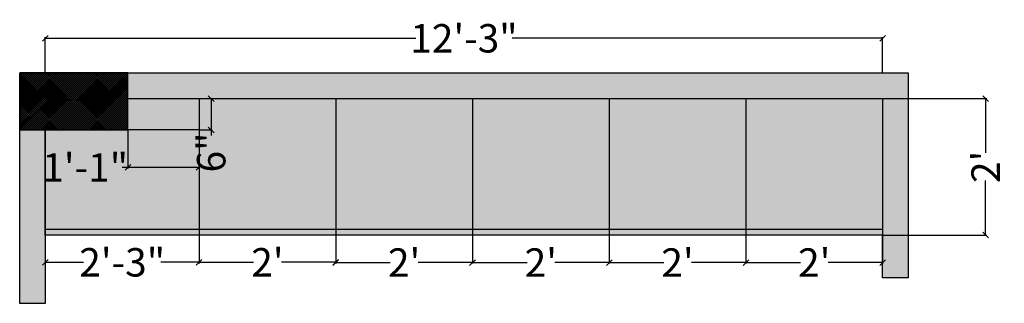
# Model space of a CAD drawing. Units: inches. Extents: x 1441 to 1633, y 516 to 722.
# Tile 2 of 2: x 1460 to 1633, y 673 to 722. Entities that reach past the tile are written whole.
import ezdxf

# ---------------------------------------------------------------- set-up
doc = ezdxf.new("R2010")
doc.units = ezdxf.units.IN
doc.header["$LTSCALE"] = 2
doc.header["$MEASUREMENT"] = 0
for name, color, linetype, lineweight in [('A-ANNO-DIMS', 2, 'Continuous', 18), ('A-FURN', 7, 'Continuous', 25), ('A-FURN-PATT', 252, 'Continuous', 13)]:
    doc.layers.add(name, color=color, linetype=linetype, lineweight=lineweight)
doc.styles.get("Standard").update_dxf_attribs({"font": 'arial.ttf'})
doc.dimstyles.get("Standard").update_dxf_attribs({"dimtxt": 5, "dimasz": 1, "dimexe": 0.18, "dimexo": 0.0625, "dimgap": 0.09, "dimtad": 0, "dimdec": 0, "dimzin": 0, "dimdsep": 46, "dimlunit": 4, "dimtxsty": 'Standard', "dimblk": 'OBLIQUE', "dimcen": 0.09, "dimadec": 0, "dimazin": 0, "dimtfac": 1, "dimtdec": 0, "dimtofl": 0, "dimtmove": 0, "dimatfit": 3, "dimldrblk": 'OBLIQUE', "dimfxl": 1, "dimtolj": 1, "dimtzin": 0, "dimarcsym": 1})

# ---------------------------------------------------------------- blocks, each defined once
blk = doc.blocks.new('_Oblique')
at = {"color": 0, "linetype": 'ByBlock', "lineweight": -2}
blk.add_line((-0.5, -0.5), (0.5, 0.5), dxfattribs=at)
blk = doc.blocks.new('*D2')
at = {"layer": 'A-ANNO-DIMS', "color": 0, "lineweight": -2, "transparency": 16777216}
for p, q in [((1464.16, 713.06), (1464.16, 719.27)), ((1611.16, 713.06), (1611.16, 719.27)), ((1464.16, 719.09), (1529.22, 719.09)), ((1611.16, 719.09), (1546.11, 719.09))]:
    blk.add_line(p, q, dxfattribs=at)
at = {"layer": 'Defpoints', "color": 0, "transparency": 16777216}
for p in [(1611.16, 719.09), (1464.16, 713), (1611.16, 713)]:
    blk.add_point(p, dxfattribs=at)
at = {"layer": 'A-ANNO-DIMS', "color": 0, "lineweight": -2, "transparency": 16777216, "rotation": 180}
blk.add_blockref('_Oblique', (1464.16, 719.09), dxfattribs=at)
at = {"layer": 'A-ANNO-DIMS', "color": 0, "lineweight": -2, "transparency": 16777216}
blk.add_blockref('_Oblique', (1611.16, 719.09), dxfattribs=at)
at = {"layer": 'A-ANNO-DIMS', "color": 0, "transparency": 16777216, "insert": (1537.66, 719.09), "char_height": 5, "attachment_point": 5}
blk.add_mtext('\\A1;12\'-3"', dxfattribs=at)
blk = doc.blocks.new('*D25')
at = {"layer": 'A-ANNO-DIMS', "color": 0, "lineweight": -2, "transparency": 16777216}
for p, q in [((1464.16, 685.44), (1464.16, 679.53)), ((1491.16, 685.44), (1491.16, 679.53)), ((1464.16, 679.71), (1470.88, 679.71)), ((1491.16, 679.71), (1484.44, 679.71))]:
    blk.add_line(p, q, dxfattribs=at)
at = {"layer": 'Defpoints', "color": 0, "transparency": 16777216}
for p in [(1464.16, 685.5), (1491.16, 685.5), (1491.16, 679.71)]:
    blk.add_point(p, dxfattribs=at)
at = {"layer": 'A-ANNO-DIMS', "color": 0, "lineweight": -2, "transparency": 16777216, "rotation": 180}
blk.add_blockref('_Oblique', (1464.16, 679.71), dxfattribs=at)
at = {"layer": 'A-ANNO-DIMS', "color": 0, "lineweight": -2, "transparency": 16777216}
blk.add_blockref('_Oblique', (1491.16, 679.71), dxfattribs=at)
at = {"layer": 'A-ANNO-DIMS', "color": 0, "transparency": 16777216, "insert": (1477.66, 679.71), "char_height": 5, "attachment_point": 5}
blk.add_mtext('\\A1;2\'-3"', dxfattribs=at)
blk = doc.blocks.new('*D26')
at = {"layer": 'A-ANNO-DIMS', "color": 0, "lineweight": -2, "transparency": 16777216}
for p, q in [((1515.16, 685.44), (1515.16, 679.53)), ((1491.16, 679.78), (1491.16, 679.89)), ((1491.16, 679.71), (1500.73, 679.71)), ((1515.16, 679.71), (1505.6, 679.71))]:
    blk.add_line(p, q, dxfattribs=at)
at = {"layer": 'Defpoints', "color": 0, "transparency": 16777216}
for p in [(1515.16, 685.5), (1491.16, 679.71), (1515.16, 679.71)]:
    blk.add_point(p, dxfattribs=at)
at = {"layer": 'A-ANNO-DIMS', "color": 0, "lineweight": -2, "transparency": 16777216, "rotation": 180}
blk.add_blockref('_Oblique', (1491.16, 679.71), dxfattribs=at)
at = {"layer": 'A-ANNO-DIMS', "color": 0, "lineweight": -2, "transparency": 16777216}
blk.add_blockref('_Oblique', (1515.16, 679.71), dxfattribs=at)
at = {"layer": 'A-ANNO-DIMS', "color": 0, "transparency": 16777216, "insert": (1503.16, 679.71), "char_height": 5, "attachment_point": 5}
blk.add_mtext("\\A1;2'", dxfattribs=at)
blk = doc.blocks.new('*D27')
at = {"layer": 'A-ANNO-DIMS', "color": 0, "lineweight": -2, "transparency": 16777216}
for p, q in [((1539.16, 685.44), (1539.16, 679.49)), ((1515.16, 679.67), (1524.73, 679.67)), ((1515.16, 679.65), (1515.16, 679.49)), ((1539.16, 679.67), (1529.6, 679.67))]:
    blk.add_line(p, q, dxfattribs=at)
at = {"layer": 'Defpoints', "color": 0, "transparency": 16777216}
for p in [(1539.16, 685.5), (1515.16, 679.71), (1515.16, 679.67)]:
    blk.add_point(p, dxfattribs=at)
at = {"layer": 'A-ANNO-DIMS', "color": 0, "lineweight": -2, "transparency": 16777216, "rotation": 180}
blk.add_blockref('_Oblique', (1515.16, 679.67), dxfattribs=at)
at = {"layer": 'A-ANNO-DIMS', "color": 0, "lineweight": -2, "transparency": 16777216}
blk.add_blockref('_Oblique', (1539.16, 679.67), dxfattribs=at)
at = {"layer": 'A-ANNO-DIMS', "color": 0, "transparency": 16777216, "insert": (1527.16, 679.67), "char_height": 5, "attachment_point": 5}
blk.add_mtext("\\A1;2'", dxfattribs=at)
blk = doc.blocks.new('*D28')
at = {"layer": 'A-ANNO-DIMS', "color": 0, "lineweight": -2, "transparency": 16777216}
for p, q in [((1539.16, 685.44), (1539.16, 679.49)), ((1563.16, 685.44), (1563.16, 679.49)), ((1539.16, 679.67), (1548.73, 679.67)), ((1563.16, 679.67), (1553.6, 679.67))]:
    blk.add_line(p, q, dxfattribs=at)
at = {"layer": 'Defpoints', "color": 0, "transparency": 16777216}
for p in [(1539.16, 685.5), (1563.16, 685.5), (1563.16, 679.67)]:
    blk.add_point(p, dxfattribs=at)
at = {"layer": 'A-ANNO-DIMS', "color": 0, "lineweight": -2, "transparency": 16777216, "rotation": 180}
blk.add_blockref('_Oblique', (1539.16, 679.67), dxfattribs=at)
at = {"layer": 'A-ANNO-DIMS', "color": 0, "lineweight": -2, "transparency": 16777216}
blk.add_blockref('_Oblique', (1563.16, 679.67), dxfattribs=at)
at = {"layer": 'A-ANNO-DIMS', "color": 0, "transparency": 16777216, "insert": (1551.16, 679.67), "char_height": 5, "attachment_point": 5}
blk.add_mtext("\\A1;2'", dxfattribs=at)
blk = doc.blocks.new('*D29')
at = {"layer": 'A-ANNO-DIMS', "color": 0, "lineweight": -2, "transparency": 16777216}
for p, q in [((1563.16, 685.44), (1563.16, 679.49)), ((1587.16, 685.44), (1587.16, 679.49)), ((1563.16, 679.67), (1572.73, 679.67)), ((1587.16, 679.67), (1577.6, 679.67))]:
    blk.add_line(p, q, dxfattribs=at)
at = {"layer": 'Defpoints', "color": 0, "transparency": 16777216}
for p in [(1563.16, 685.5), (1587.16, 685.5), (1587.16, 679.67)]:
    blk.add_point(p, dxfattribs=at)
at = {"layer": 'A-ANNO-DIMS', "color": 0, "lineweight": -2, "transparency": 16777216, "rotation": 180}
blk.add_blockref('_Oblique', (1563.16, 679.67), dxfattribs=at)
at = {"layer": 'A-ANNO-DIMS', "color": 0, "lineweight": -2, "transparency": 16777216}
blk.add_blockref('_Oblique', (1587.16, 679.67), dxfattribs=at)
at = {"layer": 'A-ANNO-DIMS', "color": 0, "transparency": 16777216, "insert": (1575.16, 679.67), "char_height": 5, "attachment_point": 5}
blk.add_mtext("\\A1;2'", dxfattribs=at)
blk = doc.blocks.new('*D30')
at = {"layer": 'A-ANNO-DIMS', "color": 0, "lineweight": -2, "transparency": 16777216}
for p, q in [((1587.16, 685.44), (1587.16, 679.49)), ((1611.16, 685.44), (1611.16, 679.49)), ((1587.16, 679.67), (1596.73, 679.67)), ((1611.16, 679.67), (1601.6, 679.67))]:
    blk.add_line(p, q, dxfattribs=at)
at = {"layer": 'Defpoints', "color": 0, "transparency": 16777216}
for p in [(1587.16, 685.5), (1611.16, 685.5), (1611.16, 679.67)]:
    blk.add_point(p, dxfattribs=at)
at = {"layer": 'A-ANNO-DIMS', "color": 0, "lineweight": -2, "transparency": 16777216, "rotation": 180}
blk.add_blockref('_Oblique', (1587.16, 679.67), dxfattribs=at)
at = {"layer": 'A-ANNO-DIMS', "color": 0, "lineweight": -2, "transparency": 16777216}
blk.add_blockref('_Oblique', (1611.16, 679.67), dxfattribs=at)
at = {"layer": 'A-ANNO-DIMS', "color": 0, "transparency": 16777216, "insert": (1599.16, 679.67), "char_height": 5, "attachment_point": 5}
blk.add_mtext("\\A1;2'", dxfattribs=at)
blk = doc.blocks.new('*D31')
at = {"layer": 'A-ANNO-DIMS', "color": 0, "lineweight": -2, "transparency": 16777216}
for p, q in [((1611.23, 708.5), (1629.43, 708.5)), ((1629.25, 708.5), (1629.25, 698.93)), ((1629.25, 684.5), (1629.25, 694.07)), ((1611.23, 684.5), (1629.43, 684.5))]:
    blk.add_line(p, q, dxfattribs=at)
at = {"layer": 'Defpoints', "color": 0, "transparency": 16777216}
for p in [(1611.16, 708.5), (1611.16, 684.5), (1629.25, 684.5)]:
    blk.add_point(p, dxfattribs=at)
at = {"layer": 'A-ANNO-DIMS', "color": 0, "lineweight": -2, "transparency": 16777216}
for p, rotation in [((1629.25, 708.5), 90), ((1629.25, 684.5), 270)]:
    blk.add_blockref('_Oblique', p, dxfattribs=dict(at, rotation=rotation))
at = {"layer": 'A-ANNO-DIMS', "color": 0, "transparency": 16777216, "insert": (1629.25, 696.5), "char_height": 5, "attachment_point": 5, "rotation": 90}
blk.add_mtext("\\A1;2'", dxfattribs=at)
blk = doc.blocks.new('*D32')
at = {"layer": 'A-ANNO-DIMS', "color": 0, "lineweight": -2, "transparency": 16777216}
for p, q in [((1478.66, 702.94), (1478.66, 696.21)), ((1491.16, 702.94), (1491.16, 696.21)), ((1478.66, 696.39), (1477.66, 696.39)), ((1491.16, 696.39), (1478.66, 696.39))]:
    blk.add_line(p, q, dxfattribs=at)
at = {"layer": 'Defpoints', "color": 0, "transparency": 16777216}
for p in [(1478.66, 703), (1491.16, 703), (1478.66, 696.39)]:
    blk.add_point(p, dxfattribs=at)
at = {"layer": 'A-ANNO-DIMS', "color": 0, "lineweight": -2, "transparency": 16777216, "rotation": 180}
blk.add_blockref('_Oblique', (1478.66, 696.39), dxfattribs=at)
at = {"layer": 'A-ANNO-DIMS', "color": 0, "lineweight": -2, "transparency": 16777216}
blk.add_blockref('_Oblique', (1491.16, 696.39), dxfattribs=at)
at = {"layer": 'A-ANNO-DIMS', "color": 0, "transparency": 16777216, "insert": (1471.16, 696.39), "char_height": 5, "attachment_point": 5}
blk.add_mtext('\\A1;1\'-1"', dxfattribs=at)
blk = doc.blocks.new('*D33')
at = {"layer": 'A-ANNO-DIMS', "color": 0, "lineweight": -2, "transparency": 16777216}
for p, q in [((1491.23, 708.5), (1493.46, 708.5)), ((1493.28, 708.5), (1493.28, 703)), ((1491.23, 703), (1493.46, 703)), ((1493.28, 703), (1493.28, 702))]:
    blk.add_line(p, q, dxfattribs=at)
at = {"layer": 'Defpoints', "color": 0, "transparency": 16777216}
for p in [(1491.16, 708.5), (1491.16, 703), (1493.28, 703)]:
    blk.add_point(p, dxfattribs=at)
at = {"layer": 'A-ANNO-DIMS', "color": 0, "lineweight": -2, "transparency": 16777216}
for p, rotation in [((1493.28, 708.5), 90), ((1493.28, 703), 270)]:
    blk.add_blockref('_Oblique', p, dxfattribs=dict(at, rotation=rotation))
at = {"layer": 'A-ANNO-DIMS', "color": 0, "transparency": 16777216, "insert": (1493.28, 699.02), "char_height": 5, "attachment_point": 5, "rotation": 90}
blk.add_mtext('\\A1;6"', dxfattribs=at)

msp = doc.modelspace()

# ---------------------------------------------------------------- hatches: boundary and pattern name
at = {"layer": 'A-FURN-PATT'}
h = msp.add_hatch(dxfattribs=at)
h.set_pattern_fill('ANSI37', color=256, scale=2)
h.set_pattern_definition([(45, (43.05178, -183.31212), (-0.176776695, 0.176776695), []), (135, (43.05178, -183.31212), (-0.176776695, -0.176776695), [])])
h.paths.add_polyline_path([(1478.66, 703), (1478.66, 713), (1459.66, 713), (1459.66, 703)])
h = msp.add_hatch(color=256, dxfattribs=at)
h.dxf.hatch_style = 1
h.paths.add_polyline_path([(1611.16, 708.5), (1611.16, 684.5), (1611.16, 677), (1615.66, 677), (1615.66, 713), (1611.16, 713), (1478.66, 713), (1478.66, 708.5)])
h.paths.add_polyline_path([(1464.16, 703), (1459.66, 703), (1459.66, 672.5), (1464.16, 672.5), (1464.16, 684.5)])
h = msp.add_hatch(color=256, dxfattribs=at)
h.dxf.hatch_style = 1
h.paths.add_polyline_path([(1491.16, 703), (1478.66, 703), (1464.16, 703), (1464.16, 685.5), (1491.16, 685.5)])
h.paths.add_polyline_path([(1491.16, 708.5), (1478.66, 708.5), (1478.66, 703), (1491.16, 703)])
h.paths.add_polyline_path([(1462.74, 695.19), (1479.15, 695.19), (1479.15, 705.49), (1462.74, 705.49)], flags=9)
h = msp.add_hatch(color=256, dxfattribs=at)
h.dxf.hatch_style = 1
h.paths.add_polyline_path([(1491.16, 708.5), (1478.66, 708.5), (1478.66, 703), (1491.16, 703)])
h.paths.add_polyline_path([(1491.16, 703), (1478.66, 703), (1464.16, 703), (1464.16, 685.5), (1491.16, 685.5)])
h.paths.add_polyline_path([(1515.16, 708.5), (1491.16, 708.5), (1491.16, 703), (1491.16, 685.5), (1515.16, 685.5)])
h.paths.add_polyline_path([(1539.16, 708.5), (1515.16, 708.5), (1515.16, 685.5), (1539.16, 685.5)])
h.paths.add_polyline_path([(1563.16, 708.5), (1539.16, 708.5), (1539.16, 685.5), (1563.16, 685.5)])
h.paths.add_polyline_path([(1587.16, 708.5), (1563.16, 708.5), (1563.16, 685.5), (1587.16, 685.5)])
h.paths.add_polyline_path([(1611.16, 708.5), (1587.16, 708.5), (1587.16, 685.5), (1611.16, 685.5)])
h.paths.add_polyline_path([(1611.16, 685.5), (1587.16, 685.5), (1587.16, 684.5), (1611.16, 684.5)])
h.paths.add_polyline_path([(1587.16, 685.5), (1563.16, 685.5), (1563.16, 684.5), (1587.16, 684.5)])
h.paths.add_polyline_path([(1563.16, 685.5), (1539.16, 685.5), (1539.16, 684.5), (1563.16, 684.5)])
h.paths.add_polyline_path([(1539.16, 685.5), (1515.16, 685.5), (1515.16, 684.5), (1539.16, 684.5)])
h.paths.add_polyline_path([(1515.16, 685.5), (1491.16, 685.5), (1491.16, 684.5), (1515.16, 684.5)])
h.paths.add_polyline_path([(1491.16, 685.5), (1464.16, 685.5), (1464.16, 684.5), (1491.16, 684.5)])

# ---------------------------------------------------------------- linework, layer by layer
at = {"layer": 'A-FURN'}
for p, q in [((1459.66, 708.5), (1459.66, 713)), ((1459.66, 713), (1464.16, 713)), ((1464.16, 713), (1611.16, 713)), ((1611.16, 713), (1615.66, 713)), ((1615.66, 713), (1615.66, 677)), ((1459.66, 672.5), (1459.66, 708.5)), ((1478.66, 708.5), (1611.16, 708.5)), ((1491.16, 708.5), (1491.16, 684.5)), ((1515.16, 708.5), (1515.16, 684.5)), ((1539.16, 708.5), (1539.16, 684.5)), ((1563.16, 708.5), (1563.16, 684.5)), ((1587.16, 708.5), (1587.16, 684.5)), ((1611.16, 708.5), (1611.16, 684.5)), ((1464.16, 684.5), (1464.16, 703)), ((1464.16, 703), (1464.16, 684.5)), ((1611.16, 685.5), (1464.16, 685.5)), ((1611.16, 684.5), (1464.16, 684.5)), ((1464.16, 684.5), (1464.16, 672.5)), ((1611.16, 677), (1611.16, 684.5)), ((1615.66, 677), (1611.16, 677)), ((1464.16, 672.5), (1459.66, 672.5))]:
    msp.add_line(p, q, dxfattribs=at)
for points in [[(1459.66, 713), (1459.66, 703), (1478.66, 703), (1478.66, 713)], [(1478.66, 708.5), (1491.16, 708.5), (1491.16, 703), (1478.66, 703)]]:
    msp.add_lwpolyline(points, close=True, dxfattribs=at)

# ---------------------------------------------------------------- dimensions: what is measured, and where the dimension line sits
at = {"layer": 'A-ANNO-DIMS'}
for base, p1, p2, picture, middle in [((1611.16, 719.09), (1464.16, 713), (1611.16, 713), '*D2', (1537.66, 719.09)), ((1478.66288514, 696.39008131), (1491.16288514, 703.00006995), (1478.66288514, 703.00006995), '*D32', (1471.162585, 696.39008131)), ((1491.16, 679.71), (1464.16, 685.5), (1491.16, 685.5), '*D25', (1477.66, 679.71)), ((1515.16, 679.71), (1491.16, 679.71), (1515.16, 685.5), '*D26', (1503.16, 679.71)), ((1515.16, 679.67), (1539.16, 685.5), (1515.16, 679.71), '*D27', (1527.16, 679.67)), ((1563.16, 679.67), (1539.16, 685.5), (1563.16, 685.5), '*D28', (1551.16, 679.67)), ((1587.16, 679.67), (1563.16, 685.5), (1587.16, 685.5), '*D29', (1575.16, 679.67)), ((1611.16, 679.67), (1587.16, 685.5), (1611.16, 685.5), '*D30', (1599.16, 679.67))]:
    dim = msp.add_linear_dim(base=base, p1=p1, p2=p2, dimstyle='Standard', override={"dimclrd": 0, "dimclre": 0, "dimclrt": 0}, dxfattribs=at)
    dim.commit()
    dim.dimension.update_dxf_attribs({"geometry": picture, "text_midpoint": middle})
for base, p1, p2, picture, middle in [((1493.27968773, 703.00006995), (1491.16288514, 708.50006995), (1491.16288514, 703.00006995), '*D33', (1493.27968773, 699.02296218)), ((1629.25, 684.5), (1611.16, 708.5), (1611.16, 684.5), '*D31', (1629.25, 696.5))]:
    dim = msp.add_linear_dim(base=base, p1=p1, p2=p2, angle=90, dimstyle='Standard', override={"dimclrd": 0, "dimclre": 0, "dimclrt": 0}, dxfattribs=at)
    dim.commit()
    dim.dimension.update_dxf_attribs({"geometry": picture, "text_midpoint": middle})

doc.saveas('drawing.dxf')
